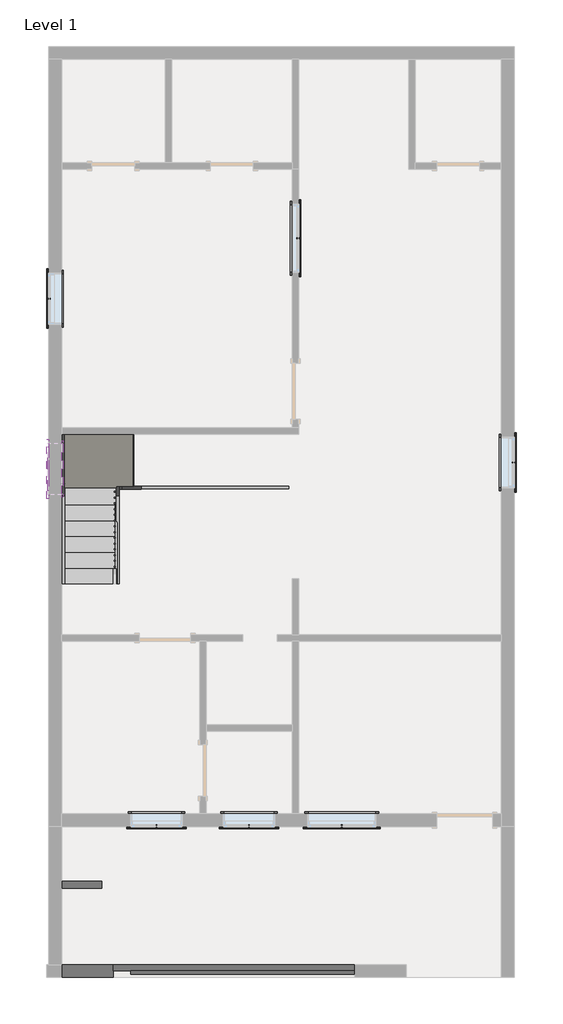
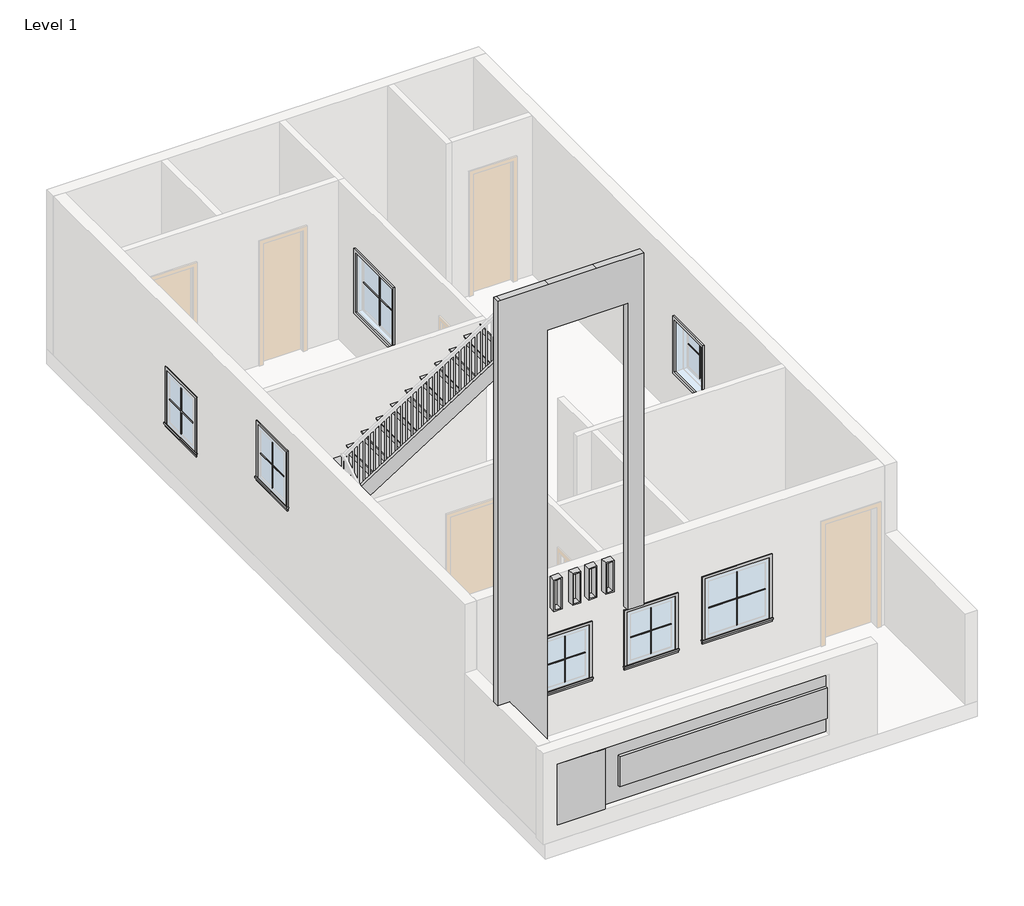
# One storey, part 2 of 2: 23 proxies, 5 members, 2 stair flights, 1 railing, 1 slab.
"""IFC4 building model written with IfcOpenShell, lengths in millimetres."""

from ifc_helpers import new_model, si_unit, point, frame, frame_2d, origin, origin_with_axes, place, context, project, spatial, polyline, circle_curve, ellipse_curve, trimmed, segment, composite_curve, outline, extrude, transform, mapped, element, save
from ifc_brep_helpers import plane_surface, cylinder_surface, advanced_brep
from components import generic_models_1_generic_models_1_d955dbe1, generic_models_2_generic_models_2_f62d3e83, muntin_pattern_2x2_muntin_pattern_2x2_5e50c346, muntin_pattern_2x2_muntin_pattern_2x2_cef8da4c, muntin_pattern_2x2_muntin_pattern_2x2_8235f178, muntin_pattern_2x2_muntin_pattern_2x2_3e21365d, trim_window_exterior_flat_with_sill_0e7a59f4, trim_window_exterior_flat_with_sill_ac84ebb5, trim_window_exterior_flat_with_sill_7cfdd449, trim_window_exterior_flat_with_sill_1a1a26d5, trim_window_interior_flat_picture_frame_9adb9ca0, trim_window_interior_flat_picture_frame_caf2db4f, trim_window_interior_flat_picture_frame_f1e0b15b, trim_window_interior_flat_picture_frame_dc353545, non_monolithic_landing_ccb861af, stair_flight_bb9b06f6, stair_flight_d3d59df2

model = new_model("IFC4")

# Units and contexts
model_context = context("Model", 3, world=origin())
ifc_project = project(units=[si_unit("LENGTHUNIT", "METRE", prefix="MILLI")], contexts=[model_context])

# Site, building, storey
site = spatial("IfcSite", under=ifc_project)
building = spatial("IfcBuilding", under=site)
storey = spatial("IfcBuildingStorey", under=building, Name="Level 1", Elevation=0.0)

# Proxies
placement = place(None, origin())
generic_models_1_generic_models_1_shape = generic_models_1_generic_models_1_d955dbe1(model_context)
element("IfcBuildingElementProxy", 1, Name="Generic Models 1 : Generic Models 1", ObjectType="Generic Models 1 : Generic Models 1", at=placement, inside=storey, context=model_context, shape_type="MappedRepresentation", body=[
    mapped(generic_models_1_generic_models_1_shape, transform((0.0, 0.0, 0.0), x_axis=(1.0, 0.0, 0.0), y_axis=(0.0, 1.0, 0.0), z_axis=(0.0, 0.0, 1.0))),
])
generic_models_2_generic_models_2_shape = generic_models_2_generic_models_2_f62d3e83(model_context)
element("IfcBuildingElementProxy", 2, Name="Generic Models 2 : Generic Models 2", ObjectType="Generic Models 2 : Generic Models 2", at=placement, inside=storey, context=model_context, shape_type="MappedRepresentation", body=[
    mapped(generic_models_2_generic_models_2_shape, transform((0.0, 0.0, 0.0), x_axis=(1.0, 0.0, 0.0), y_axis=(0.0, 1.0, 0.0), z_axis=(0.0, 0.0, 1.0))),
])
muntin_pattern_2x2_muntin_pattern_2x2_shape = muntin_pattern_2x2_muntin_pattern_2x2_5e50c346(model_context)
element("IfcBuildingElementProxy", 3, Name="Muntin Pattern_2x2 : Muntin Pattern_2x2", ObjectType="Muntin Pattern_2x2 : Muntin Pattern_2x2", at=placement, inside=storey, context=model_context, shape_type="MappedRepresentation", body=[
    mapped(muntin_pattern_2x2_muntin_pattern_2x2_shape, transform((-10378.6167709, -3243.6387867, 984.25), x_axis=(1.0, 0.0, 0.0), y_axis=(0.0, 1.0, 0.0), z_axis=(0.0, 0.0, 1.0))),
])
element("IfcBuildingElementProxy", 4, Name="Muntin Pattern_2x2 : Muntin Pattern_2x2", ObjectType="Muntin Pattern_2x2 : Muntin Pattern_2x2", at=placement, inside=storey, context=model_context, shape_type="MappedRepresentation", body=[
    mapped(muntin_pattern_2x2_muntin_pattern_2x2_shape, transform((-12016.9167709, -3243.6387867, 984.25), x_axis=(1.0, 0.0, 0.0), y_axis=(0.0, 1.0, 0.0), z_axis=(0.0, 0.0, 1.0))),
])
muntin_pattern_2x2_muntin_pattern_2x2_2_shape = muntin_pattern_2x2_muntin_pattern_2x2_cef8da4c(model_context)
element("IfcBuildingElementProxy", 5, Name="Muntin Pattern_2x2 : Muntin Pattern_2x2", ObjectType="Muntin Pattern_2x2 : Muntin Pattern_2x2", at=placement, inside=storey, context=model_context, shape_type="MappedRepresentation", body=[
    mapped(muntin_pattern_2x2_muntin_pattern_2x2_2_shape, transform((-8740.3167709, -3243.6387867, 984.25), x_axis=(1.0, 0.0, 0.0), y_axis=(0.0, 1.0, 0.0), z_axis=(0.0, 0.0, 1.0))),
])
muntin_pattern_2x2_muntin_pattern_2x2_3_shape = muntin_pattern_2x2_muntin_pattern_2x2_8235f178(model_context)
element("IfcBuildingElementProxy", 6, Name="Muntin Pattern_2x2 : Muntin Pattern_2x2", ObjectType="Muntin Pattern_2x2 : Muntin Pattern_2x2", at=placement, inside=storey, context=model_context, shape_type="MappedRepresentation", body=[
    mapped(muntin_pattern_2x2_muntin_pattern_2x2_3_shape, transform((-9511.8417709, 7148.1362133, 984.25), x_axis=(0.0, -1.0, 0.0), y_axis=(1.0, 0.0, 0.0), z_axis=(0.0, 0.0, 1.0))),
])
muntin_pattern_2x2_muntin_pattern_2x2_4_shape = muntin_pattern_2x2_muntin_pattern_2x2_3e21365d(model_context)
element("IfcBuildingElementProxy", 7, Name="Muntin Pattern_2x2 : Muntin Pattern_2x2", ObjectType="Muntin Pattern_2x2 : Muntin Pattern_2x2", at=placement, inside=storey, context=model_context, shape_type="MappedRepresentation", body=[
    mapped(muntin_pattern_2x2_muntin_pattern_2x2_4_shape, transform((-5701.8417709, 3185.7362133, 984.25), x_axis=(0.0, -1.0, 0.0), y_axis=(1.0, 0.0, 0.0), z_axis=(0.0, 0.0, 1.0))),
])
element("IfcBuildingElementProxy", 8, Name="Muntin Pattern_2x2 : Muntin Pattern_2x2", ObjectType="Muntin Pattern_2x2 : Muntin Pattern_2x2", at=placement, inside=storey, context=model_context, shape_type="MappedRepresentation", body=[
    mapped(muntin_pattern_2x2_muntin_pattern_2x2_4_shape, transform((-13912.3917709, 3071.4362133, 1723.6670763), x_axis=(0.0, 1.0, 0.0), y_axis=(-1.0, 0.0, 0.0), z_axis=(0.0, 0.0, 1.0))),
])
element("IfcBuildingElementProxy", 9, Name="Muntin Pattern_2x2 : Muntin Pattern_2x2", ObjectType="Muntin Pattern_2x2 : Muntin Pattern_2x2", at=placement, inside=storey, context=model_context, shape_type="MappedRepresentation", body=[
    mapped(muntin_pattern_2x2_muntin_pattern_2x2_4_shape, transform((-13912.3917709, 6081.3362133, 984.25), x_axis=(0.0, 1.0, 0.0), y_axis=(-1.0, 0.0, 0.0), z_axis=(0.0, 0.0, 1.0))),
])
trim_window_exterior_flat_with_sill_shape = trim_window_exterior_flat_with_sill_0e7a59f4(model_context)
element("IfcBuildingElementProxy", 10, Name="Trim-Window-Exterior-Flat : with Sill", ObjectType="Trim-Window-Exterior-Flat : with Sill", at=placement, inside=storey, context=model_context, shape_type="MappedRepresentation", body=[
    mapped(trim_window_exterior_flat_with_sill_shape, transform((-10378.6167709, -3253.1637867, 1981.2), x_axis=(-1.0, 0.0, 0.0), y_axis=(0.0, 0.0, -1.0), z_axis=(0.0, -1.0, 0.0))),
])
element("IfcBuildingElementProxy", 11, Name="Trim-Window-Exterior-Flat : with Sill", ObjectType="Trim-Window-Exterior-Flat : with Sill", at=placement, inside=storey, context=model_context, shape_type="MappedRepresentation", body=[
    mapped(trim_window_exterior_flat_with_sill_shape, transform((-12016.9167709, -3253.1637867, 1981.2), x_axis=(-1.0, 0.0, 0.0), y_axis=(0.0, 0.0, -1.0), z_axis=(0.0, -1.0, 0.0))),
])
trim_window_exterior_flat_with_sill_2_shape = trim_window_exterior_flat_with_sill_ac84ebb5(model_context)
element("IfcBuildingElementProxy", 12, Name="Trim-Window-Exterior-Flat : with Sill", ObjectType="Trim-Window-Exterior-Flat : with Sill", at=placement, inside=storey, context=model_context, shape_type="MappedRepresentation", body=[
    mapped(trim_window_exterior_flat_with_sill_2_shape, transform((-8740.3167709, -3253.1637867, 2133.6), x_axis=(-1.0, 0.0, 0.0), y_axis=(0.0, 0.0, -1.0), z_axis=(0.0, -1.0, 0.0))),
])
trim_window_exterior_flat_with_sill_3_shape = trim_window_exterior_flat_with_sill_7cfdd449(model_context)
element("IfcBuildingElementProxy", 13, Name="Trim-Window-Exterior-Flat : with Sill", ObjectType="Trim-Window-Exterior-Flat : with Sill", at=placement, inside=storey, context=model_context, shape_type="MappedRepresentation", body=[
    mapped(trim_window_exterior_flat_with_sill_3_shape, transform((-9502.3167709, 7148.1362133, 2133.6), x_axis=(0.0, 1.0, 0.0), y_axis=(0.0, 0.0, 1.0), z_axis=(1.0, 0.0, 0.0))),
])
trim_window_exterior_flat_with_sill_4_shape = trim_window_exterior_flat_with_sill_1a1a26d5(model_context)
element("IfcBuildingElementProxy", 14, Name="Trim-Window-Exterior-Flat : with Sill", ObjectType="Trim-Window-Exterior-Flat : with Sill", at=placement, inside=storey, context=model_context, shape_type="MappedRepresentation", body=[
    mapped(trim_window_exterior_flat_with_sill_4_shape, transform((-5692.3167709, 3185.7362133, 1981.2), x_axis=(0.0, 1.0, 0.0), y_axis=(0.0, 0.0, 1.0), z_axis=(1.0, 0.0, 0.0))),
])
element("IfcBuildingElementProxy", 15, Name="Trim-Window-Exterior-Flat : with Sill", ObjectType="Trim-Window-Exterior-Flat : with Sill", at=placement, inside=storey, context=model_context, shape_type="MappedRepresentation", body=[
    mapped(trim_window_exterior_flat_with_sill_4_shape, transform((-13921.9167709, 3071.4362133, 2720.6170763), x_axis=(0.0, -1.0, 0.0), y_axis=(0.0, 0.0, 1.0), z_axis=(-1.0, 0.0, 0.0))),
])
element("IfcBuildingElementProxy", 16, Name="Trim-Window-Exterior-Flat : with Sill", ObjectType="Trim-Window-Exterior-Flat : with Sill", at=placement, inside=storey, context=model_context, shape_type="MappedRepresentation", body=[
    mapped(trim_window_exterior_flat_with_sill_4_shape, transform((-13921.9167709, 6081.3362133, 1981.2), x_axis=(0.0, -1.0, 0.0), y_axis=(0.0, 0.0, 1.0), z_axis=(-1.0, 0.0, 0.0))),
])
trim_window_interior_flat_picture_frame_shape = trim_window_interior_flat_picture_frame_9adb9ca0(model_context)
element("IfcBuildingElementProxy", 17, Name="Trim-Window-Interior-Flat : Picture Frame", ObjectType="Trim-Window-Interior-Flat : Picture Frame", at=placement, inside=storey, context=model_context, shape_type="MappedRepresentation", body=[
    mapped(trim_window_interior_flat_picture_frame_shape, transform((-10378.6167709, -3024.5637867, 1981.2), x_axis=(1.0, 0.0, 0.0), y_axis=(0.0, 0.0, -1.0), z_axis=(0.0, 1.0, 0.0))),
])
element("IfcBuildingElementProxy", 18, Name="Trim-Window-Interior-Flat : Picture Frame", ObjectType="Trim-Window-Interior-Flat : Picture Frame", at=placement, inside=storey, context=model_context, shape_type="MappedRepresentation", body=[
    mapped(trim_window_interior_flat_picture_frame_shape, transform((-12016.9167709, -3024.5637867, 1981.2), x_axis=(1.0, 0.0, 0.0), y_axis=(0.0, 0.0, -1.0), z_axis=(0.0, 1.0, 0.0))),
])
trim_window_interior_flat_picture_frame_2_shape = trim_window_interior_flat_picture_frame_caf2db4f(model_context)
element("IfcBuildingElementProxy", 19, Name="Trim-Window-Interior-Flat : Picture Frame", ObjectType="Trim-Window-Interior-Flat : Picture Frame", at=placement, inside=storey, context=model_context, shape_type="MappedRepresentation", body=[
    mapped(trim_window_interior_flat_picture_frame_2_shape, transform((-8740.3167709, -3024.5637867, 2133.6), x_axis=(1.0, 0.0, 0.0), y_axis=(0.0, 0.0, -1.0), z_axis=(0.0, 1.0, 0.0))),
])
trim_window_interior_flat_picture_frame_3_shape = trim_window_interior_flat_picture_frame_f1e0b15b(model_context)
element("IfcBuildingElementProxy", 20, Name="Trim-Window-Interior-Flat : Picture Frame", ObjectType="Trim-Window-Interior-Flat : Picture Frame", at=placement, inside=storey, context=model_context, shape_type="MappedRepresentation", body=[
    mapped(trim_window_interior_flat_picture_frame_3_shape, transform((-9616.6167709, 7148.1362133, 2133.6), x_axis=(0.0, -1.0, 0.0), y_axis=(0.0, 0.0, 1.0), z_axis=(-1.0, 0.0, 0.0))),
])
trim_window_interior_flat_picture_frame_4_shape = trim_window_interior_flat_picture_frame_dc353545(model_context)
element("IfcBuildingElementProxy", 21, Name="Trim-Window-Interior-Flat : Picture Frame", ObjectType="Trim-Window-Interior-Flat : Picture Frame", at=placement, inside=storey, context=model_context, shape_type="MappedRepresentation", body=[
    mapped(trim_window_interior_flat_picture_frame_4_shape, transform((-5920.9167709, 3185.7362133, 1981.2), x_axis=(0.0, -1.0, 0.0), y_axis=(0.0, 0.0, 1.0), z_axis=(-1.0, 0.0, 0.0))),
])
element("IfcBuildingElementProxy", 22, Name="Trim-Window-Interior-Flat : Picture Frame", ObjectType="Trim-Window-Interior-Flat : Picture Frame", at=placement, inside=storey, context=model_context, shape_type="MappedRepresentation", body=[
    mapped(trim_window_interior_flat_picture_frame_4_shape, transform((-13693.3167709, 3071.4362133, 2720.6170763), x_axis=(0.0, 1.0, 0.0), y_axis=(0.0, 0.0, 1.0), z_axis=(1.0, 0.0, 0.0))),
])
element("IfcBuildingElementProxy", 23, Name="Trim-Window-Interior-Flat : Picture Frame", ObjectType="Trim-Window-Interior-Flat : Picture Frame", at=placement, inside=storey, context=model_context, shape_type="MappedRepresentation", body=[
    mapped(trim_window_interior_flat_picture_frame_4_shape, transform((-13693.3167709, 6081.3362133, 1981.2), x_axis=(0.0, 1.0, 0.0), y_axis=(0.0, 0.0, 1.0), z_axis=(1.0, 0.0, 0.0))),
])

# Members
element("IfcMember", 24, ObjectType="Stringer - 2\" Width", at=placement, inside=storey, context=model_context, shape_type="SweptSolid", body=[
    extrude(outline(polyline([(1039.4362133, 0.0), (1039.4362133, 215.0106437), (2777.1052018, 1320.8), (2865.8631712, 1016.0), (1269.2917427, 0.0), (1039.4362133, 0.0)])), frame((-13693.3167709, 0.0, 0.0), z_axis=(1.0, 0.0, 0.0), x_axis=(0.0, 1.0, 0.0)), (0.0, 0.0, 1.0), 50.8),
])
element("IfcMember", 25, ObjectType="Stringer - 2\" Width", at=placement, inside=storey, context=model_context, shape_type="SweptSolid", body=[
    extrude(outline(polyline([(1039.4362133, 0.0), (1039.4362133, 215.0106437), (2766.6362133, 1314.1379164), (2766.6362133, 952.8555722), (1269.2917427, 0.0), (1039.4362133, 0.0)])), frame((-12728.1167709, 0.0, 0.0), z_axis=(1.0, 0.0, 0.0), x_axis=(0.0, 1.0, 0.0)), (0.0, 0.0, 1.0), 50.8),
])
element("IfcMember", 26, ObjectType="Stringer - 2\" Width", at=placement, inside=storey, context=model_context, shape_type="SweptSolid", body=[
    extrude(outline(polyline([(1320.8, -12666.8477824), (1016.0, -12578.0898129), (2876.3282995, -9654.7167709), (3237.6106437, -9654.7167709), (1320.8, -12666.8477824)])), frame((0.0, 2715.8362133, 0.0), z_axis=(0.0, 1.0, 0.0), x_axis=(0.0, 0.0, 1.0)), (0.0, 0.0, 1.0), 50.8),
])
element("IfcMember", 27, ObjectType="Stringer - 2\" Width", at=placement, inside=storey, context=model_context, shape_type="SweptSolid", body=[
    extrude(outline(polyline([(3681.0362133, 1320.8), (3681.0362133, 1016.0), (2865.8631712, 1016.0), (2777.1052018, 1320.8), (3681.0362133, 1320.8)])), frame((-13693.3167709, 0.0, 0.0), z_axis=(1.0, 0.0, 0.0), x_axis=(0.0, 1.0, 0.0)), (0.0, 0.0, 1.0), 50.8),
])
element("IfcMember", 28, ObjectType="Stringer - 2\" Width", at=placement, inside=storey, context=model_context, shape_type="SweptSolid", body=[
    extrude(outline(polyline([(1320.8, -12677.3167709), (1016.0, -12677.3167709), (1016.0, -12578.0898129), (1320.8, -12666.8477824), (1320.8, -12677.3167709)])), frame((0.0, 2715.8362133, 0.0), z_axis=(0.0, 1.0, 0.0), x_axis=(0.0, 0.0, 1.0)), (0.0, 0.0, 1.0), 50.8),
])

# Railing
element("IfcRailing", 29, ObjectType="Handrail - Pipe", at=placement, inside=storey, context=model_context, shape_type="SolidModel", body=[
    advanced_brep(
    [(-12709.0667709, 1039.4362133, 895.35), (-12747.1667709, 1039.4362133, 895.35), (-12709.0667709, 2722.1862133, 895.35), (-12747.1667709, 2760.2862133, 895.35), (-9680.1167709, 2722.1862133, 895.35), (-9680.1167709, 2760.2862133, 895.35)],
    [
        (0, 1, circle_curve(frame((-12728.1167709, 1039.4362133, 895.35), z_axis=(0.0, -1.0, 0.0), x_axis=(-1.0, 0.0, 0.0)), 19.05)),
        (1, 0, circle_curve(frame((-12728.1167709, 1039.4362133, 895.35), z_axis=(0.0, -1.0, 0.0), x_axis=(-1.0, 0.0, 0.0)), 19.05)),
        (0, 2),
        (2, 3, ellipse_curve(frame((-12728.1167709, 2741.2362133, 895.35), z_axis=(-0.7071067811865491, -0.7071067811865458, 0.0), x_axis=(0.7071067811865457, -0.7071067811865492, 0.0)), 26.9407684, 19.05)),
        (3, 1),
        (3, 2, ellipse_curve(frame((-12728.1167709, 2741.2362133, 895.35), z_axis=(-0.7071067811865491, -0.7071067811865458, 0.0), x_axis=(0.7071067811865457, -0.7071067811865492, 0.0)), 26.9407684, 19.05)),
        (4, 5, circle_curve(frame((-9680.1167709, 2741.2362133, 895.35), z_axis=(1.0, 0.0, 0.0), x_axis=(0.0, 1.0, 0.0)), 19.05)),
        (5, 4, circle_curve(frame((-9680.1167709, 2741.2362133, 895.35), z_axis=(1.0, 0.0, 0.0), x_axis=(0.0, 1.0, 0.0)), 19.05)),
        (2, 4),
        (5, 3),
    ],
    [
        plane_surface(frame((-12728.1167709, 1039.4362133, 914.4), z_axis=(0.0, -1.0, 0.0), x_axis=(0.0, 0.0, 1.0))),
        cylinder_surface(frame((-12728.1167709, 1039.4362133, 895.35), z_axis=(0.0, -1.0, 0.0), x_axis=(-1.0, 0.0, 0.0)), 19.05),
        plane_surface(frame((-9680.1167709, 2741.2362133, 914.4), z_axis=(1.0, 0.0, 0.0), x_axis=(0.0, 1.0, 0.0))),
        cylinder_surface(frame((-12728.1167709, 2741.2362133, 895.35), z_axis=(-1.0, 0.0, 0.0), x_axis=(0.0, 1.0, 0.0)), 19.05),
    ],
    [
        (0, [[1, 2]]),
        (1, [[-1, 3, 4, 5]]),
        (1, [[-2, -5, 6, -3]]),
        (2, [[7, 8]]),
        (3, [[-4, 9, -8, 10]]),
        (3, [[-6, -10, -7, -9]]),
    ],
),
    advanced_brep(
    [(-12740.8167709, 1039.4362133, 749.3), (-12715.4167709, 1039.4362133, 749.3), (-12740.8167709, 2753.9362133, 749.3), (-12715.4167709, 2728.5362133, 749.3), (-9680.1167709, 2753.9362133, 749.3), (-9680.1167709, 2728.5362133, 749.3)],
    [
        (0, 1, circle_curve(frame((-12728.1167709, 1039.4362133, 749.3), z_axis=(0.0, -1.0, 0.0), x_axis=(1.0, 0.0, 0.0)), 12.7)),
        (1, 0, circle_curve(frame((-12728.1167709, 1039.4362133, 749.3), z_axis=(0.0, -1.0, 0.0), x_axis=(1.0, 0.0, 0.0)), 12.7)),
        (0, 2),
        (2, 3, ellipse_curve(frame((-12728.1167709, 2741.2362133, 749.3), z_axis=(-0.7071067811865491, -0.7071067811865458, 0.0), x_axis=(0.7071067811865457, -0.7071067811865492, 0.0)), 17.9605122, 12.7)),
        (3, 1),
        (3, 2, ellipse_curve(frame((-12728.1167709, 2741.2362133, 749.3), z_axis=(-0.7071067811865491, -0.7071067811865458, 0.0), x_axis=(0.7071067811865457, -0.7071067811865492, 0.0)), 17.9605122, 12.7)),
        (4, 5, circle_curve(frame((-9680.1167709, 2741.2362133, 749.3), z_axis=(1.0, 0.0, 0.0), x_axis=(0.0, -1.0, 0.0)), 12.7)),
        (5, 4, circle_curve(frame((-9680.1167709, 2741.2362133, 749.3), z_axis=(1.0, 0.0, 0.0), x_axis=(0.0, -1.0, 0.0)), 12.7)),
        (2, 4),
        (5, 3),
    ],
    [
        plane_surface(frame((-12728.1167709, 1039.4362133, 762.0), z_axis=(0.0, -1.0, 0.0), x_axis=(0.0, 0.0, 1.0))),
        cylinder_surface(frame((-12728.1167709, 1039.4362133, 749.3), z_axis=(0.0, -1.0, 0.0), x_axis=(1.0, 0.0, 0.0)), 12.7),
        plane_surface(frame((-9680.1167709, 2741.2362133, 762.0), z_axis=(1.0, 0.0, 0.0), x_axis=(0.0, 1.0, 0.0))),
        cylinder_surface(frame((-12728.1167709, 2741.2362133, 749.3), z_axis=(-1.0, 0.0, 0.0), x_axis=(0.0, -1.0, 0.0)), 12.7),
    ],
    [
        (0, [[1, 2]]),
        (1, [[-1, 3, 4, 5]]),
        (1, [[-2, -5, 6, -3]]),
        (2, [[7, 8]]),
        (3, [[-4, 9, -8, 10]]),
        (3, [[-6, -10, -7, -9]]),
    ],
),
    advanced_brep(
    [(-12740.8167709, 1039.4362133, 596.9), (-12715.4167709, 1039.4362133, 596.9), (-12740.8167709, 2753.9362133, 596.9), (-12715.4167709, 2728.5362133, 596.9), (-9680.1167709, 2753.9362133, 596.9), (-9680.1167709, 2728.5362133, 596.9)],
    [
        (0, 1, circle_curve(frame((-12728.1167709, 1039.4362133, 596.9), z_axis=(0.0, -1.0, 0.0), x_axis=(1.0, 0.0, 0.0)), 12.7)),
        (1, 0, circle_curve(frame((-12728.1167709, 1039.4362133, 596.9), z_axis=(0.0, -1.0, 0.0), x_axis=(1.0, 0.0, 0.0)), 12.7)),
        (0, 2),
        (2, 3, ellipse_curve(frame((-12728.1167709, 2741.2362133, 596.9), z_axis=(-0.7071067811865491, -0.7071067811865458, 0.0), x_axis=(0.7071067811865457, -0.7071067811865492, 0.0)), 17.9605122, 12.7)),
        (3, 1),
        (3, 2, ellipse_curve(frame((-12728.1167709, 2741.2362133, 596.9), z_axis=(-0.7071067811865491, -0.7071067811865458, 0.0), x_axis=(0.7071067811865457, -0.7071067811865492, 0.0)), 17.9605122, 12.7)),
        (4, 5, circle_curve(frame((-9680.1167709, 2741.2362133, 596.9), z_axis=(1.0, 0.0, 0.0), x_axis=(0.0, -1.0, 0.0)), 12.7)),
        (5, 4, circle_curve(frame((-9680.1167709, 2741.2362133, 596.9), z_axis=(1.0, 0.0, 0.0), x_axis=(0.0, -1.0, 0.0)), 12.7)),
        (2, 4),
        (5, 3),
    ],
    [
        plane_surface(frame((-12728.1167709, 1039.4362133, 609.6), z_axis=(0.0, -1.0, 0.0), x_axis=(0.0, 0.0, 1.0))),
        cylinder_surface(frame((-12728.1167709, 1039.4362133, 596.9), z_axis=(0.0, -1.0, 0.0), x_axis=(1.0, 0.0, 0.0)), 12.7),
        plane_surface(frame((-9680.1167709, 2741.2362133, 609.6), z_axis=(1.0, 0.0, 0.0), x_axis=(0.0, 1.0, 0.0))),
        cylinder_surface(frame((-12728.1167709, 2741.2362133, 596.9), z_axis=(-1.0, 0.0, 0.0), x_axis=(0.0, -1.0, 0.0)), 12.7),
    ],
    [
        (0, [[1, 2]]),
        (1, [[-1, 3, 4, 5]]),
        (1, [[-2, -5, 6, -3]]),
        (2, [[7, 8]]),
        (3, [[-4, 9, -8, 10]]),
        (3, [[-6, -10, -7, -9]]),
    ],
),
    advanced_brep(
    [(-12740.8167709, 1039.4362133, 444.5), (-12715.4167709, 1039.4362133, 444.5), (-12740.8167709, 2753.9362133, 444.5), (-12715.4167709, 2728.5362133, 444.5), (-9680.1167709, 2753.9362133, 444.5), (-9680.1167709, 2728.5362133, 444.5)],
    [
        (0, 1, circle_curve(frame((-12728.1167709, 1039.4362133, 444.5), z_axis=(0.0, -1.0, 0.0), x_axis=(1.0, 0.0, 0.0)), 12.7)),
        (1, 0, circle_curve(frame((-12728.1167709, 1039.4362133, 444.5), z_axis=(0.0, -1.0, 0.0), x_axis=(1.0, 0.0, 0.0)), 12.7)),
        (0, 2),
        (2, 3, ellipse_curve(frame((-12728.1167709, 2741.2362133, 444.5), z_axis=(-0.7071067811865491, -0.7071067811865458, 0.0), x_axis=(0.7071067811865457, -0.7071067811865492, 0.0)), 17.9605122, 12.7)),
        (3, 1),
        (3, 2, ellipse_curve(frame((-12728.1167709, 2741.2362133, 444.5), z_axis=(-0.7071067811865491, -0.7071067811865458, 0.0), x_axis=(0.7071067811865457, -0.7071067811865492, 0.0)), 17.9605122, 12.7)),
        (4, 5, circle_curve(frame((-9680.1167709, 2741.2362133, 444.5), z_axis=(1.0, 0.0, 0.0), x_axis=(0.0, -1.0, 0.0)), 12.7)),
        (5, 4, circle_curve(frame((-9680.1167709, 2741.2362133, 444.5), z_axis=(1.0, 0.0, 0.0), x_axis=(0.0, -1.0, 0.0)), 12.7)),
        (2, 4),
        (5, 3),
    ],
    [
        plane_surface(frame((-12728.1167709, 1039.4362133, 457.2), z_axis=(0.0, -1.0, 0.0), x_axis=(0.0, 0.0, 1.0))),
        cylinder_surface(frame((-12728.1167709, 1039.4362133, 444.5), z_axis=(0.0, -1.0, 0.0), x_axis=(1.0, 0.0, 0.0)), 12.7),
        plane_surface(frame((-9680.1167709, 2741.2362133, 457.2), z_axis=(1.0, 0.0, 0.0), x_axis=(0.0, 1.0, 0.0))),
        cylinder_surface(frame((-12728.1167709, 2741.2362133, 444.5), z_axis=(-1.0, 0.0, 0.0), x_axis=(0.0, -1.0, 0.0)), 12.7),
    ],
    [
        (0, [[1, 2]]),
        (1, [[-1, 3, 4, 5]]),
        (1, [[-2, -5, 6, -3]]),
        (2, [[7, 8]]),
        (3, [[-4, 9, -8, 10]]),
        (3, [[-6, -10, -7, -9]]),
    ],
),
    advanced_brep(
    [(-12740.8167709, 1039.4362133, 292.1), (-12715.4167709, 1039.4362133, 292.1), (-12740.8167709, 2753.9362133, 292.1), (-12715.4167709, 2728.5362133, 292.1), (-9680.1167709, 2753.9362133, 292.1), (-9680.1167709, 2728.5362133, 292.1)],
    [
        (0, 1, circle_curve(frame((-12728.1167709, 1039.4362133, 292.1), z_axis=(0.0, -1.0, 0.0), x_axis=(1.0, 0.0, 0.0)), 12.7)),
        (1, 0, circle_curve(frame((-12728.1167709, 1039.4362133, 292.1), z_axis=(0.0, -1.0, 0.0), x_axis=(1.0, 0.0, 0.0)), 12.7)),
        (0, 2),
        (2, 3, ellipse_curve(frame((-12728.1167709, 2741.2362133, 292.1), z_axis=(-0.7071067811865491, -0.7071067811865458, 0.0), x_axis=(0.7071067811865457, -0.7071067811865492, 0.0)), 17.9605122, 12.7)),
        (3, 1),
        (3, 2, ellipse_curve(frame((-12728.1167709, 2741.2362133, 292.1), z_axis=(-0.7071067811865491, -0.7071067811865458, 0.0), x_axis=(0.7071067811865457, -0.7071067811865492, 0.0)), 17.9605122, 12.7)),
        (4, 5, circle_curve(frame((-9680.1167709, 2741.2362133, 292.1), z_axis=(1.0, 0.0, 0.0), x_axis=(0.0, -1.0, 0.0)), 12.7)),
        (5, 4, circle_curve(frame((-9680.1167709, 2741.2362133, 292.1), z_axis=(1.0, 0.0, 0.0), x_axis=(0.0, -1.0, 0.0)), 12.7)),
        (2, 4),
        (5, 3),
    ],
    [
        plane_surface(frame((-12728.1167709, 1039.4362133, 304.8), z_axis=(0.0, -1.0, 0.0), x_axis=(0.0, 0.0, 1.0))),
        cylinder_surface(frame((-12728.1167709, 1039.4362133, 292.1), z_axis=(0.0, -1.0, 0.0), x_axis=(1.0, 0.0, 0.0)), 12.7),
        plane_surface(frame((-9680.1167709, 2741.2362133, 304.8), z_axis=(1.0, 0.0, 0.0), x_axis=(0.0, 1.0, 0.0))),
        cylinder_surface(frame((-12728.1167709, 2741.2362133, 292.1), z_axis=(-1.0, 0.0, 0.0), x_axis=(0.0, -1.0, 0.0)), 12.7),
    ],
    [
        (0, [[1, 2]]),
        (1, [[-1, 3, 4, 5]]),
        (1, [[-2, -5, 6, -3]]),
        (2, [[7, 8]]),
        (3, [[-4, 9, -8, 10]]),
        (3, [[-6, -10, -7, -9]]),
    ],
),
    advanced_brep(
    [(-12740.8167709, 1039.4362133, 139.7), (-12715.4167709, 1039.4362133, 139.7), (-12740.8167709, 2753.9362133, 139.7), (-12715.4167709, 2728.5362133, 139.7), (-9680.1167709, 2753.9362133, 139.7), (-9680.1167709, 2728.5362133, 139.7)],
    [
        (0, 1, circle_curve(frame((-12728.1167709, 1039.4362133, 139.7), z_axis=(0.0, -1.0, 0.0), x_axis=(1.0, 0.0, 0.0)), 12.7)),
        (1, 0, circle_curve(frame((-12728.1167709, 1039.4362133, 139.7), z_axis=(0.0, -1.0, 0.0), x_axis=(1.0, 0.0, 0.0)), 12.7)),
        (0, 2),
        (2, 3, ellipse_curve(frame((-12728.1167709, 2741.2362133, 139.7), z_axis=(-0.7071067811865491, -0.7071067811865458, 0.0), x_axis=(0.7071067811865457, -0.7071067811865492, 0.0)), 17.9605122, 12.7)),
        (3, 1),
        (3, 2, ellipse_curve(frame((-12728.1167709, 2741.2362133, 139.7), z_axis=(-0.7071067811865491, -0.7071067811865458, 0.0), x_axis=(0.7071067811865457, -0.7071067811865492, 0.0)), 17.9605122, 12.7)),
        (4, 5, circle_curve(frame((-9680.1167709, 2741.2362133, 139.7), z_axis=(1.0, 0.0, 0.0), x_axis=(0.0, -1.0, 0.0)), 12.7)),
        (5, 4, circle_curve(frame((-9680.1167709, 2741.2362133, 139.7), z_axis=(1.0, 0.0, 0.0), x_axis=(0.0, -1.0, 0.0)), 12.7)),
        (2, 4),
        (5, 3),
    ],
    [
        plane_surface(frame((-12728.1167709, 1039.4362133, 152.4), z_axis=(0.0, -1.0, 0.0), x_axis=(0.0, 0.0, 1.0))),
        cylinder_surface(frame((-12728.1167709, 1039.4362133, 139.7), z_axis=(0.0, -1.0, 0.0), x_axis=(1.0, 0.0, 0.0)), 12.7),
        plane_surface(frame((-9680.1167709, 2741.2362133, 152.4), z_axis=(1.0, 0.0, 0.0), x_axis=(0.0, 1.0, 0.0))),
        cylinder_surface(frame((-12728.1167709, 2741.2362133, 139.7), z_axis=(-1.0, 0.0, 0.0), x_axis=(0.0, -1.0, 0.0)), 12.7),
    ],
    [
        (0, [[1, 2]]),
        (1, [[-1, 3, 4, 5]]),
        (1, [[-2, -5, 6, -3]]),
        (2, [[7, 8]]),
        (3, [[-4, 9, -8, 10]]),
        (3, [[-6, -10, -7, -9]]),
    ],
),
    extrude(outline(composite_curve([segment(trimmed(circle_curve(frame_2d((-10289.7167709, 2741.2362133)), 12.7), [point((-10289.7167709, 2753.9362133))], [point((-10289.7167709, 2728.5362133))], False, "CARTESIAN"), True, "CONTINUOUS"), segment(trimmed(circle_curve(frame_2d((-10289.7167709, 2741.2362133)), 12.7), [point((-10289.7167709, 2728.5362133))], [point((-10289.7167709, 2753.9362133))], False, "CARTESIAN"), True, "CONTINUOUS")], self_intersect=False)), origin_with_axes(), (0.0, 0.0, 1.0), 876.3),
    extrude(outline(composite_curve([segment(trimmed(circle_curve(frame_2d((-11508.9167709, 2741.2362133)), 12.7), [point((-11508.9167709, 2753.9362133))], [point((-11508.9167709, 2728.5362133))], False, "CARTESIAN"), True, "CONTINUOUS"), segment(trimmed(circle_curve(frame_2d((-11508.9167709, 2741.2362133)), 12.7), [point((-11508.9167709, 2728.5362133))], [point((-11508.9167709, 2753.9362133))], False, "CARTESIAN"), True, "CONTINUOUS")], self_intersect=False)), origin_with_axes(), (0.0, 0.0, 1.0), 876.3),
    extrude(outline(composite_curve([segment(trimmed(circle_curve(frame_2d((-12728.1167709, 2258.6362133)), 12.7), [point((-12740.8167709, 2258.6362133))], [point((-12715.4167709, 2258.6362133))], False, "CARTESIAN"), True, "CONTINUOUS"), segment(trimmed(circle_curve(frame_2d((-12728.1167709, 2258.6362133)), 12.7), [point((-12715.4167709, 2258.6362133))], [point((-12740.8167709, 2258.6362133))], False, "CARTESIAN"), True, "CONTINUOUS")], self_intersect=False)), origin_with_axes(), (0.0, 0.0, 1.0), 876.3),
    extrude(outline(composite_curve([segment(trimmed(circle_curve(frame_2d((-12728.1167709, 2741.2362133)), 12.7), [point((-12740.8167709, 2741.2362133))], [point((-12715.4167709, 2741.2362133))], False, "CARTESIAN"), True, "CONTINUOUS"), segment(trimmed(circle_curve(frame_2d((-12728.1167709, 2741.2362133)), 12.7), [point((-12715.4167709, 2741.2362133))], [point((-12740.8167709, 2741.2362133))], False, "CARTESIAN"), True, "CONTINUOUS")], self_intersect=False)), origin_with_axes(), (0.0, 0.0, 1.0), 876.3),
    extrude(outline(composite_curve([segment(trimmed(circle_curve(frame_2d((-9692.8167709, 2741.2362133)), 12.7), [point((-9692.8167709, 2753.9362133))], [point((-9692.8167709, 2728.5362133))], False, "CARTESIAN"), True, "CONTINUOUS"), segment(trimmed(circle_curve(frame_2d((-9692.8167709, 2741.2362133)), 12.7), [point((-9692.8167709, 2728.5362133))], [point((-9692.8167709, 2753.9362133))], False, "CARTESIAN"), True, "CONTINUOUS")], self_intersect=False)), origin_with_axes(), (0.0, 0.0, 1.0), 876.3),
    extrude(outline(composite_curve([segment(trimmed(circle_curve(frame_2d((-12728.1167709, 1052.1362133)), 12.7), [point((-12740.8167709, 1052.1362133))], [point((-12715.4167709, 1052.1362133))], False, "CARTESIAN"), True, "CONTINUOUS"), segment(trimmed(circle_curve(frame_2d((-12728.1167709, 1052.1362133)), 12.7), [point((-12715.4167709, 1052.1362133))], [point((-12740.8167709, 1052.1362133))], False, "CARTESIAN"), True, "CONTINUOUS")], self_intersect=False)), origin_with_axes(), (0.0, 0.0, 1.0), 876.3),
])

# Slab
non_monolithic_landing_shape = non_monolithic_landing_ccb861af(model_context)
element("IfcSlab", 30, ObjectType="Non-Monolithic Landing", at=placement, inside=storey, context=model_context, shape_type="MappedRepresentation", body=[
    mapped(non_monolithic_landing_shape, transform((0.0, 0.0, 0.0), x_axis=(1.0, 0.0, 0.0), y_axis=(0.0, 1.0, 0.0), z_axis=(0.0, 0.0, 1.0))),
])

# Stair flights
stair_flight_shape = stair_flight_bb9b06f6(model_context)
element("IfcStairFlight", 31, ObjectType="2\" Tread 1\" Nosing 1/4\" Riser", at=placement, inside=storey, context=model_context, shape_type="MappedRepresentation", body=[
    mapped(stair_flight_shape, transform((0.0, 0.0, 0.0), x_axis=(1.0, 0.0, 0.0), y_axis=(0.0, 1.0, 0.0), z_axis=(0.0, 0.0, 1.0))),
])
stair_flight_2_shape = stair_flight_d3d59df2(model_context)
element("IfcStairFlight", 32, ObjectType="2\" Tread 1\" Nosing 1/4\" Riser", at=placement, inside=storey, context=model_context, shape_type="MappedRepresentation", body=[
    mapped(stair_flight_2_shape, transform((0.0, 0.0, 0.0), x_axis=(1.0, 0.0, 0.0), y_axis=(0.0, 1.0, 0.0), z_axis=(0.0, 0.0, 1.0))),
])

save(model, "model.ifc")

# Revit data of these elements
# Type "Muntin Pattern_2x2 : Muntin Pattern_2x2"
#   Width [instance default] = 4' - 0"
#   Thickness = 0' - 0 1/2"
#   Height [instance default] = 4' - 0"
#   Distance = 0' - 0 3/4"
#   Interior Material [instance default] = none
#   Exterior Material [instance default] = none
#   Default Elevation = 0
# Type "Trim-Window-Exterior-Flat : with Sill"
#   Trim Width = 0' - 2 1/4"
#   Trim Thickness_Picture Frame = 0' - 1 1/4"
#   Trim Thickness_with Sill = 0' - 0 3/4"
#   Sill Thickness = 0' - 1 1/4"
#   Opening Width [instance default] = 2' - 0"
#   Opening Height [instance default] = 3' - 0"
#   Default Elevation = 4' - 0"
#   Sill = yes
#   Picture Frame = no
#   Trim Material [instance default] = none
# Type "Trim-Window-Interior-Flat : Picture Frame"
#   Trim Thickness_Picture Frame = 0' - 1 1/4"
#   Trim Width = 0' - 2 1/4"
#   Trim Thickness_with Sill = 0' - 0 3/4"
#   Sill Thickness = 0' - 1 1/4"
#   Opening Width [instance default] = 2' - 0"
#   Opening Height [instance default] = 3' - 0"
#   Default Elevation = 4' - 0"
#   Sill = no
#   Picture Frame = yes
#   Trim Material [instance default] = none
# Type "Handrail - Pipe"
#   Assembly Code = "C2010400"
#   built-in parameter 1008612 = 0.0416667 (stored number, unit not read)
#   built-in parameter 1008611 = 0.0833333 (stored number, unit not read)
#   built-in parameter 1008609 = 4 (stored number, unit not read)
#   built-in parameter 1008604 = 0.166667 (stored number, unit not read)
#   built-in parameter 1008603 = 0.166667 (stored number, unit not read)
#   Railing Height = 3' - 0"
#   built-in parameter 1008630 = 2
#   built-in parameter 1008610 = 1
#   built-in parameter 1008605 = 1
#   built-in parameter 1008618 = Baluster - Round : 1"
# Element 1 (IfcBuildingElementProxy, "Generic Models 1 : Generic Models 1")
#   Phase Created = New Construction
# Element 2 (IfcBuildingElementProxy, "Generic Models 2 : Generic Models 2")
#   Phase Created = New Construction
# Elements 3, 4, 7, 8, 9 (IfcBuildingElementProxy, "Muntin Pattern_2x2 : Muntin Pattern_2x2")
#   Width = 2' - 6 1/2"
#   Height = 3' - 0 1/2"
#   Interior Material = Wood - Stained
#   Exterior Material = Clad - White
#   Phase Created = New Construction
#   Materials on its faces: "Clad - White", "Wood - Stained"
# Elements 5, 6 (IfcBuildingElementProxy, "Muntin Pattern_2x2 : Muntin Pattern_2x2")
#   Width = 3' - 6 1/2"
#   Height = 3' - 6 1/2"
#   Interior Material = Wood - Stained
#   Exterior Material = Clad - White
#   Phase Created = New Construction
#   Materials on its faces: "Clad - White", "Wood - Stained"
# Elements 10, 11, 14, 15, 16 (IfcBuildingElementProxy, "Trim-Window-Exterior-Flat : with Sill")
#   Opening Width = 3' - 0"
#   Opening Height = 3' - 6"
#   Trim Material = Clad - White
#   Phase Created = New Construction
#   Materials on its faces: "Clad - White"
# Elements 12, 13 (IfcBuildingElementProxy, "Trim-Window-Exterior-Flat : with Sill")
#   Opening Width = 4' - 0"
#   Opening Height = 4' - 0"
#   Trim Material = Clad - White
#   Phase Created = New Construction
#   Materials on its faces: "Clad - White"
# Elements 17, 18, 21, 22, 23 (IfcBuildingElementProxy, "Trim-Window-Interior-Flat : Picture Frame")
#   Opening Width = 3' - 0"
#   Opening Height = 3' - 6"
#   Trim Material = Wood - Stained
#   Phase Created = New Construction
#   Materials on its faces: "Wood - Stained"
# Elements 19, 20 (IfcBuildingElementProxy, "Trim-Window-Interior-Flat : Picture Frame")
#   Opening Width = 4' - 0"
#   Opening Height = 4' - 0"
#   Trim Material = Wood - Stained
#   Phase Created = New Construction
#   Materials on its faces: "Wood - Stained"
# Elements 24, 25, 26, 27, 28 (IfcMember, "Stringer - 2\" Width")
#   Phase Created = New Construction
# Element 29 (IfcRailing, "Handrail - Pipe")
#   Phase Created = New Construction
# Element 30 (IfcSlab, "Non-Monolithic Landing")
#   Phase Created = New Construction
# Elements 31, 32 (IfcStairFlight, "2\" Tread 1\" Nosing 1/4\" Riser")
#   Phase Created = New Construction
# Materials
#   "Clad - White": class "Wood", colour RGB 242 242 238, transparency 0, Cost = 0
#   "Wood - Stained": class "Wood", colour RGB 224 178 126, transparency 0, Cost = 0
